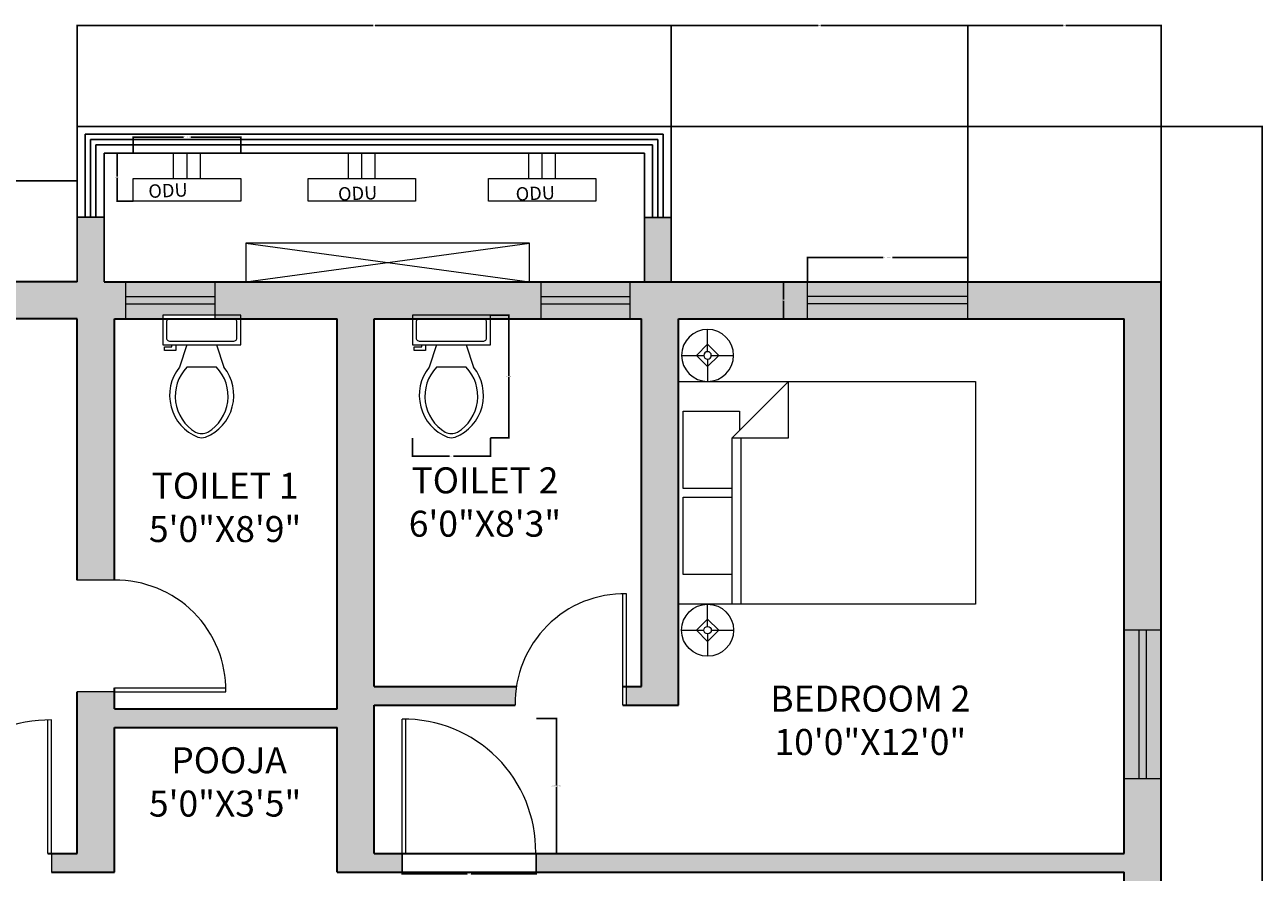
# Model space of a CAD drawing. Units: inches. Extents: x -382 to 250, y 518 to 1732.
# Tile 8 of 8: x -86 to 247, y 1504 to 1732. Entities that reach past the tile are written whole.
import ezdxf

# ---------------------------------------------------------------- set-up
doc = ezdxf.new("R2010")
doc.units = ezdxf.units.IN
doc.header["$MEASUREMENT"] = 0
for name, color, linetype, lineweight in [('A-ANNO-DIMS', 2, 'Continuous', 18), ('A-AREA-IDEN', 7, 'Continuous', 18), ('A-DOOR', 3, 'Continuous', 18), ('A-FLOR-EDGE', 7, 'Continuous', 25), ('A-FLOR-FIXT', 8, 'Continuous', 18), ('A-FLOR-SHFT', 8, 'Continuous', 18), ('A-FURN', 8, 'Continuous', 18), ('A-GLAZ', 4, 'Continuous', 18), ('A-WALL', 7, 'Continuous', 35), ('M-ANNO-TEXT', 7, 'Continuous', 13), ('M-HVAC-EQPM', 4, 'Continuous', 18)]:
    doc.layers.add(name, color=color, linetype=linetype, lineweight=lineweight)
doc.layers.add('A-GLAZ-PATT', color=143, linetype='Continuous', lineweight=13, true_color=0x7aafdf)
doc.layers.add('A-WALL-PATT', color=251, linetype='Continuous', lineweight=13, true_color=0x636466)
doc.styles.get("Standard").update_dxf_attribs({"font": 'arial.ttf'})
doc.dimstyles.get("Standard").update_dxf_attribs({"dimtxt": 0.18, "dimasz": 0.18, "dimexe": 0.18, "dimexo": 0.0625, "dimgap": 0.09, "dimtad": 0, "dimtih": 1, "dimtoh": 1, "dimdec": 4, "dimzin": 0, "dimdsep": 46, "dimtxsty": 'Standard', "dimcen": 0.09, "dimadec": 0, "dimazin": 0, "dimtfac": 1, "dimtdec": 4, "dimtofl": 0, "dimtmove": 0, "dimatfit": 3, "dimfxl": 1, "dimtolj": 1, "dimtzin": 0, "dimarcsym": 0})

# ---------------------------------------------------------------- blocks, each defined once
blk = doc.blocks.new('Bed - Queen')
for p, q in [((0, -80.00003), (0, 0)), ((0, 0), (59.99999, 0)), ((59.99999, 0), (59.99999, -80.00003)), ((7.99999, -1.2), (28.79998, -1.2)), ((7.99999, -14.4), (7.99999, -1.2)), ((28.79998, -1.2), (28.79998, -14.4)), ((31.19999, -1.2), (51.99999, -1.2)), ((31.19999, -14.4), (31.19999, -1.2)), ((51.99999, -1.2), (51.99999, -16.4)), ((0, -14.4), (44.8, -14.4)), ((59.99999, -29.6), (44.8, -14.4)), ((44.8, -14.4), (44.8, -29.6)), ((51.99999, -16.4), (46.79936, -16.4)), ((44.8, -16.8), (0, -16.8)), ((44.8, -29.6), (59.99999, -29.6)), ((59.99999, -80.00003), (0, -80.00003))]:
    blk.add_line(p, q)
blk = doc.blocks.new('Lamp - Table')
for p, q in [((0, 7), (0, 1)), ((-1, 0), (-7, 0)), ((0, 3), (-3, 0)), ((-3, 0), (0, -3)), ((3, 0), (0, 3)), ((0, -3), (3, 0)), ((1, 0), (7, 0)), ((0, -1), (0, -7))]:
    blk.add_line(p, q)
for radius in [7, 1]:
    blk.add_circle((0, 0), radius)
blk = doc.blocks.new('Toilet - top')
for p, q in [((9.5, -6), (9.5, -2)), ((-10, -8.5), (-8, -8.5)), ((-10, -9.5), (-10, -8.5)), ((-7, -9.5), (-10, -9.5)), ((-8, -8.5), (-8, -8)), ((-7, -8), (-7, -9.5)), ((-4, -8), (-6, -14)), ((4, -8), (6, -14)), ((4, -14), (-4, -14))]:
    blk.add_line(p, q)
blk.add_lwpolyline([(10.5, -8), (10.5, 0), (-10.5, 0), (-10.5, -8)], close=True)
for points in [[(-9.5, -2), (-9.5, -6)], [(8.5, -1), (-8.5, -1)], [(-8.5, -7), (8.5, -7)]]:
    blk.add_lwpolyline(points)
for centre, radius, start, end in [((-8.62, -1.88), 0.884, 81.8699, 188.1301), ((8.62, -1.88), 0.884, 351.8699, 98.1301), ((-8.62, -6.12), 0.884, 171.8699, 278.1301), ((8.62, -6.12), 0.884, 261.8699, 8.1301), ((3.52, -21.58), 12.17, 141.4691, 247.9714), ((4.2, -21.82), 11.33, 136.3677, 238.9468), ((-3.52, -21.58), 12.17, 292.0284, 38.5307), ((-4.2, -21.82), 11.33, 301.053, 43.6321), ((0, -27.88), 4, 245.7318, 294.2682), ((0, -29), 4, 254.8605, 285.1395)]:
    blk.add_arc(centre, radius, start, end)
blk = doc.blocks.new('WIN-43_2IN')
for p, q in [((0, 10), (0, 0)), ((43.2, 10), (43.2, 0)), ((0, 6), (43.2, 6)), ((0, 4), (43.2, 4))]:
    blk.add_line(p, q)
blk = doc.blocks.new('WIN-40IN')
for p, q in [((10, 40), (0, 40)), ((4, 40), (4, 0)), ((6, 40), (6, 0)), ((10, 0), (0, 0))]:
    blk.add_line(p, q)
blk = doc.blocks.new('WIN-24IN')
for p, q in [((0, 0), (0, 10)), ((24, 0), (24, 10)), ((0, 6), (24, 6)), ((0, 4), (24, 4))]:
    blk.add_line(p, q)
blk = doc.blocks.new('DOOR-SWING-36IN')
for p, q in [((-1, 0), (-1, 36)), ((0, 0), (0, 36))]:
    blk.add_line(p, q)
blk.add_arc((-0.5, 0.5), 35.5, 89.1931, 180.8069)
blk = doc.blocks.new('DOOR-SWING-30IN')
for p, q in [((0, 1), (30, 1)), ((0, 0), (30, 0))]:
    blk.add_line(p, q)
blk.add_arc((0.5, 0.5), 29.5, 359.029, 90.971)
blk = doc.blocks.new('ODU-LEDGE-MEDIUM')
for p, q in [((10.89, 6.17), (10.89, 12.93)), ((14.49, 6.17), (14.49, 12.93)), ((18.09, 6.17), (18.09, 12.93))]:
    blk.add_line(p, q)
blk.add_lwpolyline([(0, 6.17), (28.98, 6.17), (28.98, 0), (0, 0)], close=True)
blk = doc.blocks.new('DOOR-SWING-36IN-OFFSET')
for p, q in [((0, 0), (0, 36)), ((1, -0.22), (1, 36))]:
    blk.add_line(p, q)
blk.add_arc((0.5, 0.5), 35.5, 359.1931, 90.8069)
blk = doc.blocks.new('*D42')
at = {"layer": 'A-ANNO-DIMS', "color": 0, "lineweight": -2, "transparency": 16777216}
for p, q in [((39.13, 1654.07), (44.21, 1654.07)), ((44.03, 1653.89), (44.03, 1637.73)), ((44.03, 1621.2), (44.03, 1637.36)), ((39.13, 1621.02), (44.21, 1621.02))]:
    blk.add_line(p, q, dxfattribs=at)
at = {"layer": 'A-ANNO-DIMS', "color": 0, "transparency": 16777216}
for points in [[(44, 1653.89), (44.06, 1653.89), (44.03, 1654.07)], [(44, 1621.2), (44.06, 1621.2), (44.03, 1621.02)]]:
    blk.add_solid(points, dxfattribs=at)
at = {"layer": 'Defpoints', "color": 0, "transparency": 16777216}
for p in [(39.07, 1654.07), (44.03, 1654.07), (39.07, 1621.02)]:
    blk.add_point(p, dxfattribs=at)
at = {"layer": 'A-ANNO-DIMS', "color": 0, "transparency": 16777216, "insert": (44.03, 1637.55), "char_height": 0.18, "attachment_point": 5}
blk.add_mtext('\\A1;WC 33 TYP.', dxfattribs=at)
blk = doc.blocks.new('*D43')
at = {"layer": 'A-ANNO-DIMS', "color": 0, "lineweight": -2, "transparency": 16777216}
for p, q in [((18.07, 1620.96), (18.07, 1615.89)), ((39.07, 1620.96), (39.07, 1615.89)), ((18.25, 1616.07), (28.04, 1616.07)), ((38.89, 1616.07), (29.1, 1616.07))]:
    blk.add_line(p, q, dxfattribs=at)
at = {"layer": 'A-ANNO-DIMS', "color": 0, "transparency": 16777216}
for points in [[(18.25, 1616.1), (18.25, 1616.04), (18.07, 1616.07)], [(38.89, 1616.1), (38.89, 1616.04), (39.07, 1616.07)]]:
    blk.add_solid(points, dxfattribs=at)
at = {"layer": 'Defpoints', "color": 0, "transparency": 16777216}
for p in [(18.07, 1621.02), (39.07, 1621.02), (39.07, 1616.07)]:
    blk.add_point(p, dxfattribs=at)
at = {"layer": 'A-ANNO-DIMS', "color": 0, "transparency": 16777216, "insert": (28.57, 1616.07), "char_height": 0.18, "attachment_point": 5}
blk.add_mtext('\\A1;21 TYP.', dxfattribs=at)
blk = doc.blocks.new('*D52')
at = {"layer": 'A-ANNO-DIMS', "color": 0, "lineweight": -2, "transparency": 16777216}
for p, q in [((-57.14, 1697.73), (-57.14, 1702.19)), ((-56.96, 1702.01), (-43.64, 1702.01)), ((-28.34, 1702.01), (-41.66, 1702.01)), ((-28.16, 1697.73), (-28.16, 1702.19))]:
    blk.add_line(p, q, dxfattribs=at)
at = {"layer": 'A-ANNO-DIMS', "color": 0, "transparency": 16777216}
for points in [[(-56.96, 1702.04), (-56.96, 1701.98), (-57.14, 1702.01)], [(-28.34, 1702.04), (-28.34, 1701.98), (-28.16, 1702.01)]]:
    blk.add_solid(points, dxfattribs=at)
at = {"layer": 'Defpoints', "color": 0, "transparency": 16777216}
for p in [(-28.16, 1702.01), (-57.14, 1697.66), (-28.16, 1697.66)]:
    blk.add_point(p, dxfattribs=at)
at = {"layer": 'A-ANNO-DIMS', "color": 0, "transparency": 16777216, "insert": (-42.65, 1702.01), "char_height": 0.18, "attachment_point": 5}
blk.add_mtext('\\A1;ODU-M 29 TYP.', dxfattribs=at)
blk = doc.blocks.new('*D53')
at = {"layer": 'A-ANNO-DIMS', "color": 0, "lineweight": -2, "transparency": 16777216}
for p, q in [((-57.2, 1697.66), (-61.67, 1697.66)), ((-61.49, 1697.48), (-61.49, 1691.38)), ((-61.49, 1684.91), (-61.49, 1691.02)), ((-57.2, 1684.73), (-61.67, 1684.73))]:
    blk.add_line(p, q, dxfattribs=at)
at = {"layer": 'A-ANNO-DIMS', "color": 0, "transparency": 16777216}
for points in [[(-61.52, 1697.48), (-61.46, 1697.48), (-61.49, 1697.66)], [(-61.52, 1684.91), (-61.46, 1684.91), (-61.49, 1684.73)]]:
    blk.add_solid(points, dxfattribs=at)
at = {"layer": 'Defpoints', "color": 0, "transparency": 16777216}
for p in [(-61.49, 1697.66), (-57.14, 1697.66), (-57.14, 1684.73)]:
    blk.add_point(p, dxfattribs=at)
at = {"layer": 'A-ANNO-DIMS', "color": 0, "transparency": 16777216, "insert": (-61.49, 1691.2), "char_height": 0.18, "attachment_point": 5}
blk.add_mtext('\\A1;13 TYP.', dxfattribs=at)
blk = doc.blocks.new('*D62')
at = {"layer": 'A-ANNO-DIMS', "color": 0, "lineweight": -2, "transparency": 16777216}
for p, q in [((51.48, 1545.42), (57.05, 1545.42)), ((56.87, 1545.24), (56.87, 1527.43)), ((56.87, 1509.25), (56.87, 1527.06)), ((51.48, 1509.07), (57.05, 1509.07))]:
    blk.add_line(p, q, dxfattribs=at)
at = {"layer": 'A-ANNO-DIMS', "color": 0, "transparency": 16777216}
for points in [[(56.84, 1545.24), (56.9, 1545.24), (56.87, 1545.42)], [(56.84, 1509.25), (56.9, 1509.25), (56.87, 1509.07)]]:
    blk.add_solid(points, dxfattribs=at)
at = {"layer": 'Defpoints', "color": 0, "transparency": 16777216}
for p in [(51.42, 1545.42), (56.87, 1545.42), (51.42, 1509.07)]:
    blk.add_point(p, dxfattribs=at)
at = {"layer": 'A-ANNO-DIMS', "color": 0, "transparency": 16777216, "insert": (56.87, 1527.24), "char_height": 0.18, "attachment_point": 5}
blk.add_mtext('\\A1;OFFSET DOOR 36 TYP.', dxfattribs=at)
blk = doc.blocks.new('*D63')
at = {"layer": 'A-ANNO-DIMS', "color": 0, "lineweight": -2, "transparency": 16777216}
for p, q in [((15.29, 1509.01), (15.29, 1503.44)), ((51.42, 1509.01), (51.42, 1503.44)), ((15.47, 1503.62), (32.82, 1503.62)), ((51.24, 1503.62), (33.88, 1503.62))]:
    blk.add_line(p, q, dxfattribs=at)
at = {"layer": 'A-ANNO-DIMS', "color": 0, "transparency": 16777216}
for points in [[(15.47, 1503.65), (15.47, 1503.59), (15.29, 1503.62)], [(51.24, 1503.65), (51.24, 1503.59), (51.42, 1503.62)]]:
    blk.add_solid(points, dxfattribs=at)
at = {"layer": 'Defpoints', "color": 0, "transparency": 16777216}
for p in [(15.29, 1509.07), (51.42, 1509.07), (51.42, 1503.62)]:
    blk.add_point(p, dxfattribs=at)
at = {"layer": 'A-ANNO-DIMS', "color": 0, "transparency": 16777216, "insert": (33.35, 1503.62), "char_height": 0.18, "attachment_point": 5}
blk.add_mtext('\\A1;36 TYP.', dxfattribs=at)
blk = doc.blocks.new('*D68')
at = {"layer": 'A-ANNO-DIMS', "color": 0, "lineweight": -2, "transparency": 16777216}
for p, q in [((124.53, 1663.13), (124.53, 1669.73)), ((124.71, 1669.55), (144.89, 1669.55)), ((167.55, 1669.55), (147.37, 1669.55)), ((167.73, 1663.13), (167.73, 1669.73))]:
    blk.add_line(p, q, dxfattribs=at)
at = {"layer": 'A-ANNO-DIMS', "color": 0, "transparency": 16777216}
for points in [[(124.71, 1669.58), (124.71, 1669.52), (124.53, 1669.55)], [(167.55, 1669.58), (167.55, 1669.52), (167.73, 1669.55)]]:
    blk.add_solid(points, dxfattribs=at)
at = {"layer": 'Defpoints', "color": 0, "transparency": 16777216}
for p in [(124.53, 1669.55), (124.53, 1663.07), (167.73, 1663.07)]:
    blk.add_point(p, dxfattribs=at)
at = {"layer": 'A-ANNO-DIMS', "color": 0, "transparency": 16777216, "insert": (146.13, 1669.55), "char_height": 0.18, "attachment_point": 5}
blk.add_mtext('\\A1;WINDOW A 43 TYP.', dxfattribs=at)
blk = doc.blocks.new('*D69')
at = {"layer": 'A-ANNO-DIMS', "color": 0, "lineweight": -2, "transparency": 16777216}
for p, q in [((124.47, 1663.07), (117.87, 1663.07)), ((118.05, 1662.89), (118.05, 1658.25)), ((118.05, 1653.25), (118.05, 1657.89)), ((124.47, 1653.07), (117.87, 1653.07))]:
    blk.add_line(p, q, dxfattribs=at)
at = {"layer": 'A-ANNO-DIMS', "color": 0, "transparency": 16777216}
for points in [[(118.02, 1662.89), (118.08, 1662.89), (118.05, 1663.07)], [(118.02, 1653.25), (118.08, 1653.25), (118.05, 1653.07)]]:
    blk.add_solid(points, dxfattribs=at)
at = {"layer": 'Defpoints', "color": 0, "transparency": 16777216}
for p in [(124.53, 1663.07), (118.05, 1653.07), (124.53, 1653.07)]:
    blk.add_point(p, dxfattribs=at)
at = {"layer": 'A-ANNO-DIMS', "color": 0, "transparency": 16777216, "insert": (118.05, 1658.07), "char_height": 0.18, "attachment_point": 5}
blk.add_mtext('\\A1;10 TYP.', dxfattribs=at)
blk = doc.blocks.new('*D87')
at = {"layer": 'A-ANNO-DIMS', "color": 0, "lineweight": -2, "transparency": 16777216}
for p, q in [((87.85, 1704.87), (247.16, 1704.87)), ((246.98, 1704.69), (246.98, 1437.22)), ((246.98, 1169.38), (246.98, 1436.85)), ((82.25, 1169.2), (247.16, 1169.2))]:
    blk.add_line(p, q, dxfattribs=at)
at = {"layer": 'A-ANNO-DIMS', "color": 0, "transparency": 16777216}
for points in [[(246.95, 1704.69), (247.01, 1704.69), (246.98, 1704.87)], [(246.95, 1169.38), (247.01, 1169.38), (246.98, 1169.2)]]:
    blk.add_solid(points, dxfattribs=at)
at = {"layer": 'Defpoints', "color": 0, "transparency": 16777216}
for p in [(87.78, 1704.87), (246.98, 1704.87), (82.19, 1169.2)]:
    blk.add_point(p, dxfattribs=at)
at = {"layer": 'A-ANNO-DIMS', "color": 0, "transparency": 16777216, "insert": (246.98, 1437.03), "char_height": 0.18, "attachment_point": 5}
blk.add_mtext('\\A1;535.7', dxfattribs=at)
blk = doc.blocks.new('*D88')
at = {"layer": 'A-ANNO-DIMS', "color": 0, "lineweight": -2, "transparency": 16777216}
for p, q in [((-202.22, 1663.13), (-202.22, 1690.45)), ((-202.04, 1690.27), (-137.5, 1690.27)), ((-72.4, 1690.27), (-136.93, 1690.27)), ((-72.22, 1663.13), (-72.22, 1690.45))]:
    blk.add_line(p, q, dxfattribs=at)
at = {"layer": 'A-ANNO-DIMS', "color": 0, "transparency": 16777216}
for points in [[(-202.04, 1690.3), (-202.04, 1690.24), (-202.22, 1690.27)], [(-72.4, 1690.3), (-72.4, 1690.24), (-72.22, 1690.27)]]:
    blk.add_solid(points, dxfattribs=at)
at = {"layer": 'Defpoints', "color": 0, "transparency": 16777216}
for p in [(-72.22, 1690.27), (-202.22, 1663.07), (-72.22, 1663.07)]:
    blk.add_point(p, dxfattribs=at)
at = {"layer": 'A-ANNO-DIMS', "color": 0, "transparency": 16777216, "insert": (-137.22, 1690.27), "char_height": 0.18, "attachment_point": 5}
blk.add_mtext('\\A1;130', dxfattribs=at)
blk = doc.blocks.new('*D89')
at = {"layer": 'A-ANNO-DIMS', "color": 0, "lineweight": -2, "transparency": 16777216}
for p, q in [((-72.22, 1704.93), (-72.22, 1732.25)), ((-72.04, 1732.07), (7.5, 1732.07)), ((87.6, 1732.07), (8.07, 1732.07)), ((87.78, 1704.93), (87.78, 1732.25))]:
    blk.add_line(p, q, dxfattribs=at)
at = {"layer": 'A-ANNO-DIMS', "color": 0, "transparency": 16777216}
for points in [[(-72.04, 1732.1), (-72.04, 1732.04), (-72.22, 1732.07)], [(87.6, 1732.1), (87.6, 1732.04), (87.78, 1732.07)]]:
    blk.add_solid(points, dxfattribs=at)
at = {"layer": 'Defpoints', "color": 0, "transparency": 16777216}
for p in [(87.78, 1732.07), (-72.22, 1704.87), (87.78, 1704.87)]:
    blk.add_point(p, dxfattribs=at)
at = {"layer": 'A-ANNO-DIMS', "color": 0, "transparency": 16777216, "insert": (7.78, 1732.07), "char_height": 0.18, "attachment_point": 5}
blk.add_mtext('\\A1;160', dxfattribs=at)
blk = doc.blocks.new('*D90')
at = {"layer": 'A-ANNO-DIMS', "color": 0, "lineweight": -2, "transparency": 16777216}
for p, q in [((87.78, 1704.93), (87.78, 1732.25)), ((87.96, 1732.07), (127.36, 1732.07)), ((167.55, 1732.07), (128.15, 1732.07)), ((167.73, 1663.13), (167.73, 1732.25))]:
    blk.add_line(p, q, dxfattribs=at)
at = {"layer": 'A-ANNO-DIMS', "color": 0, "transparency": 16777216}
for points in [[(87.96, 1732.1), (87.96, 1732.04), (87.78, 1732.07)], [(167.55, 1732.1), (167.55, 1732.04), (167.73, 1732.07)]]:
    blk.add_solid(points, dxfattribs=at)
at = {"layer": 'Defpoints', "color": 0, "transparency": 16777216}
for p in [(167.73, 1732.07), (87.78, 1704.87), (167.73, 1663.07)]:
    blk.add_point(p, dxfattribs=at)
at = {"layer": 'A-ANNO-DIMS', "color": 0, "transparency": 16777216, "insert": (127.76, 1732.07), "char_height": 0.18, "attachment_point": 5}
blk.add_mtext('\\A1;79.95', dxfattribs=at)
blk = doc.blocks.new('*D96')
at = {"layer": 'A-ANNO-DIMS', "color": 0, "lineweight": -2, "transparency": 16777216}
for p, q in [((167.73, 1663.13), (167.73, 1732.25)), ((167.91, 1732.07), (193.36, 1732.07)), ((219.6, 1732.07), (194.15, 1732.07)), ((219.78, 1663.13), (219.78, 1732.25))]:
    blk.add_line(p, q, dxfattribs=at)
at = {"layer": 'A-ANNO-DIMS', "color": 0, "transparency": 16777216}
for points in [[(167.91, 1732.1), (167.91, 1732.04), (167.73, 1732.07)], [(219.6, 1732.1), (219.6, 1732.04), (219.78, 1732.07)]]:
    blk.add_solid(points, dxfattribs=at)
at = {"layer": 'Defpoints', "color": 0, "transparency": 16777216}
for p in [(219.78, 1732.07), (167.73, 1663.07), (219.78, 1663.07)]:
    blk.add_point(p, dxfattribs=at)
at = {"layer": 'A-ANNO-DIMS', "color": 0, "transparency": 16777216, "insert": (193.76, 1732.07), "char_height": 0.18, "attachment_point": 5}
blk.add_mtext('\\A1;52.05', dxfattribs=at)

msp = doc.modelspace()

# ---------------------------------------------------------------- hatches: boundary and pattern name
at = {"layer": 'A-GLAZ-PATT'}
h = msp.add_hatch(color=256, dxfattribs=at)
h.dxf.hatch_style = 1
h.paths.add_polyline_path([(-35.1064, 1663.0687), (-59.1064, 1663.0687), (-59.1064, 1659.0687), (-35.1064, 1659.0687)])
h = msp.add_hatch(color=256, dxfattribs=at)
h.dxf.hatch_style = 1
h.paths.add_polyline_path([(76.7201, 1663.0687), (52.7201, 1663.0687), (52.7201, 1659.0687), (76.7201, 1659.0687)])
h = msp.add_hatch(color=256, dxfattribs=at)
h.dxf.hatch_style = 1
h.paths.add_polyline_path([(167.7319, 1663.0687), (149.785, 1663.0687), (124.5319, 1663.0687), (124.5319, 1659.0687), (167.7319, 1659.0687)])
h = msp.add_hatch(color=256, dxfattribs=at)
h.dxf.hatch_style = 1
h.paths.add_polyline_path([(-35.1064, 1659.0687), (-59.1064, 1659.0687), (-59.1064, 1657.0687), (-35.1064, 1657.0687)])
h = msp.add_hatch(color=256, dxfattribs=at)
h.dxf.hatch_style = 1
h.paths.add_polyline_path([(76.7201, 1659.0687), (52.7201, 1659.0687), (52.7201, 1657.0687), (76.7201, 1657.0687)])
h = msp.add_hatch(color=256, dxfattribs=at)
h.dxf.hatch_style = 1
h.paths.add_polyline_path([(167.7319, 1659.0687), (124.5319, 1659.0687), (124.5319, 1657.0687), (167.7319, 1657.0687)])
h = msp.add_hatch(color=256, dxfattribs=at)
h.dxf.hatch_style = 1
h.paths.add_polyline_path([(-35.1064, 1657.0687), (-59.1064, 1657.0687), (-59.1064, 1653.0687), (-49.1947, 1653.0687), (-49.1947, 1654.0687), (-35.1064, 1654.0687)])
h = msp.add_hatch(color=256, dxfattribs=at)
h.dxf.hatch_style = 1
h.paths.add_polyline_path([(76.7201, 1657.0687), (52.7201, 1657.0687), (52.7201, 1653.0687), (76.7201, 1653.0687)])
h = msp.add_hatch(color=256, dxfattribs=at)
h.dxf.hatch_style = 1
h.paths.add_polyline_path([(167.7319, 1657.0687), (124.5319, 1657.0687), (124.5319, 1653.0687), (167.7319, 1653.0687)])
h = msp.add_hatch(color=256, dxfattribs=at)
h.dxf.hatch_style = 1
h.paths.add_polyline_path([(213.785, 1569.2079), (209.785, 1569.2079), (209.785, 1529.2079), (213.785, 1529.2079)])
h = msp.add_hatch(color=256, dxfattribs=at)
h.dxf.hatch_style = 1
h.paths.add_polyline_path([(215.785, 1569.2079), (213.785, 1569.2079), (213.785, 1529.2079), (215.785, 1529.2079)])
h = msp.add_hatch(color=256, dxfattribs=at)
h.dxf.hatch_style = 1
h.paths.add_polyline_path([(219.785, 1569.2079), (215.785, 1569.2079), (215.785, 1529.2079), (219.785, 1529.2079)])
at = {"layer": 'A-WALL-PATT'}
h = msp.add_hatch(color=256, dxfattribs=at)
h.dxf.hatch_style = 1
h.paths.add_polyline_path([(-62.215, 1653.0687), (-59.1064, 1653.0687), (-59.1064, 1663.0687), (-65.0078, 1663.0687), (-65.0078, 1680.4388), (-72.215, 1680.4388), (-72.215, 1663.0687), (-113.7732, 1663.0687), (-113.7732, 1653.0687), (-72.215, 1653.0687), (-72.215, 1582.6793), (-62.215, 1582.6793)])
h = msp.add_hatch(color=256, dxfattribs=at)
h.dxf.hatch_style = 1
h.paths.add_polyline_path([(87.785, 1680.366), (80.5778, 1680.366), (80.5778, 1663.0687), (87.785, 1663.0687)])
h = msp.add_hatch(color=256, dxfattribs=at)
h.dxf.hatch_style = 1
h.paths.add_polyline_path([(-62.215, 1543.0687), (-2.215, 1543.0687), (-2.215, 1504.0687), (15.2853, 1504.0687), (15.2853, 1509.0687), (7.785, 1509.0687), (7.785, 1549.0687), (45.742, 1549.0687, -0.04254204), (46.083, 1554.0687), (7.785, 1554.0687), (7.785, 1653.0687), (52.7201, 1653.0687), (52.7201, 1663.0687), (7.785, 1663.0687), (-26.8096, 1663.0687), (-35.1064, 1663.0687), (-35.1064, 1653.0687), (-2.215, 1653.0687), (-2.215, 1548.0687), (-62.215, 1548.0687), (-62.215, 1552.6793), (-72.215, 1552.6793), (-72.215, 1509.0687), (-79.1204, 1509.0687), (-79.1204, 1504.0687), (-62.215, 1504.0687)])
h = msp.add_hatch(color=256, dxfattribs=at)
h.dxf.hatch_style = 1
h.paths.add_polyline_path([(89.785, 1653.0687), (124.5319, 1653.0687), (124.5319, 1663.0687), (89.785, 1663.0687), (76.7201, 1663.0687), (76.7201, 1653.0687), (79.785, 1653.0687), (79.785, 1554.0687), (75.742, 1554.0687), (75.742, 1549.0687), (89.785, 1549.0687)])
h = msp.add_hatch(color=256, dxfattribs=at)
h.dxf.hatch_style = 1
h.paths.add_polyline_path([(219.785, 1663.0687), (167.7319, 1663.0687), (167.7319, 1653.0687), (209.785, 1653.0687), (209.785, 1569.2079), (219.785, 1569.2079)])
h = msp.add_hatch(color=256, dxfattribs=at)
h.dxf.hatch_style = 1
h.paths.add_polyline_path([(219.785, 1529.2079), (209.785, 1529.2079), (209.785, 1509.0687), (51.2853, 1509.0687), (51.2853, 1504.0687), (209.785, 1504.0687), (209.785, 1489.835), (219.785, 1489.835)])

# ---------------------------------------------------------------- linework, layer by layer
at = {"layer": 'A-DOOR'}
for p, q in [((-62.215, 1582.6793), (-72.215, 1582.6793)), ((-62.215, 1552.6793), (-72.215, 1552.6793)), ((-79.1204, 1509.0687), (-79.1204, 1504.0687)), ((15.2853, 1509.2855), (15.2853, 1504.0687)), ((51.2853, 1509.2855), (51.2853, 1504.0687))]:
    msp.add_line(p, q, dxfattribs=at)
at = {"layer": 'A-FLOR-EDGE'}
for p, q in [((-72.215, 1663.0687), (-72.215, 1704.8705)), ((-72.215, 1704.8705), (87.785, 1704.8705)), ((-70.0529, 1680.366), (-70.0529, 1702.7914)), ((85.6228, 1702.7914), (-70.0529, 1702.7914)), ((85.6228, 1680.366), (85.6228, 1702.7914)), ((87.785, 1663.0687), (87.785, 1704.8705)), ((-68.6114, 1680.366), (-68.6114, 1701.35)), ((84.1814, 1701.35), (-68.6114, 1701.35)), ((-67.17, 1680.366), (-67.17, 1699.9085)), ((82.7399, 1699.9085), (-67.17, 1699.9085)), ((82.7399, 1680.366), (82.7399, 1699.9085)), ((84.1814, 1680.366), (84.1814, 1701.35)), ((-65.0078, 1663.0687), (-65.0078, 1697.6633)), ((-65.0078, 1697.6633), (80.5778, 1697.6633)), ((80.5778, 1663.0687), (80.5778, 1697.6633)), ((-72.215, 1680.4388), (-65.0078, 1680.4388)), ((80.5778, 1680.366), (87.785, 1680.366))]:
    msp.add_line(p, q, dxfattribs=at)
at = {"layer": 'A-FLOR-SHFT'}
for p, q in [((-26.8096, 1663.0687), (49.5868, 1673.4832)), ((-26.8096, 1673.4832), (49.5868, 1663.0687))]:
    msp.add_line(p, q, dxfattribs=at)
msp.add_lwpolyline([(-26.8096, 1663.0687), (49.5868, 1663.0687), (49.5868, 1673.4832), (-26.8096, 1673.4832)], close=True, dxfattribs=at)
at = {"layer": 'A-WALL'}
for p, q in [((-72.215, 1663.0687), (-202.215, 1663.0687)), ((-65.0078, 1663.0687), (7.785, 1663.0687)), ((7.785, 1663.0687), (89.785, 1663.0687)), ((89.785, 1663.0687), (150.3243, 1663.0687)), ((149.785, 1663.0687), (219.785, 1663.0687)), ((219.785, 1489.835), (219.785, 1663.0687)), ((-72.215, 1653.0687), (-192.215, 1653.0687)), ((-72.215, 1582.6793), (-72.215, 1653.0687)), ((-62.215, 1653.0687), (-2.215, 1653.0687)), ((-62.215, 1582.6793), (-62.215, 1653.0687)), ((-2.215, 1548.0687), (-2.215, 1653.0687)), ((7.785, 1653.0687), (79.785, 1653.0687)), ((7.785, 1554.0687), (7.785, 1653.0687)), ((79.785, 1554.0687), (79.785, 1653.0687)), ((89.785, 1549.0687), (89.785, 1653.0687)), ((89.785, 1653.0687), (209.785, 1653.0687)), ((209.785, 1509.0687), (209.785, 1653.0687)), ((-72.215, 1509.0687), (-72.215, 1552.6793)), ((-62.215, 1548.0687), (-62.215, 1553.6793)), ((7.785, 1554.0687), (46.083, 1554.0687)), ((74.742, 1554.0687), (79.785, 1554.0687)), ((7.785, 1509.0687), (7.785, 1549.0687)), ((7.785, 1549.0687), (45.742, 1549.0687)), ((74.742, 1549.0687), (89.785, 1549.0687)), ((-62.215, 1548.0687), (-2.215, 1548.0687)), ((-62.215, 1504.0687), (-62.215, 1543.0687)), ((-62.215, 1543.0687), (-2.215, 1543.0687)), ((-2.215, 1504.0687), (-2.215, 1543.0687)), ((-80.1204, 1509.0687), (-72.215, 1509.0687)), ((7.785, 1509.0687), (209.785, 1509.0687)), ((-79.1204, 1504.0687), (-62.215, 1504.0687)), ((-2.215, 1504.0687), (209.785, 1504.0687)), ((209.785, 1488.835), (209.785, 1504.0687))]:
    msp.add_line(p, q, dxfattribs=at)
at = {"layer": 'M-HVAC-EQPM'}
msp.add_lwpolyline([(-10.0519, 1690.9042), (18.9263, 1690.9042), (18.9263, 1684.7324), (-10.0519, 1684.7324)], close=True, dxfattribs=at)

# ---------------------------------------------------------------- block references
at = {"layer": 'A-DOOR'}
for name, p in [('DOOR-SWING-30IN', (-62.215, 1552.6793)), ('DOOR-SWING-36IN', (-79.1204, 1509.0687)), ('DOOR-SWING-36IN-OFFSET', (15.2853, 1509.2855))]:
    msp.add_blockref(name, p, dxfattribs=at)
at = {"layer": 'A-DOOR', "rotation": 89.99999999999991}
msp.add_blockref('DOOR-SWING-30IN', (75.742, 1549.0687), dxfattribs=at)
at = {"layer": 'A-FLOR-FIXT'}
for p in [(-38.6947, 1654.0687), (28.572, 1654.0687)]:
    msp.add_blockref('Toilet - top', p, dxfattribs=at)
at = {"layer": 'A-FURN', "xscale": -1, "rotation": 90}
msp.add_blockref('Lamp - Table', (97.5964, 1643.2304), dxfattribs=at)
at = {"layer": 'A-FURN', "rotation": 90}
for name, p in [('Bed - Queen', (89.785, 1576.2304)), ('Lamp - Table', (97.5964, 1569.2304))]:
    msp.add_blockref(name, p, dxfattribs=at)
at = {"layer": 'A-GLAZ'}
for name, p in [('WIN-24IN', (-59.106, 1653.069)), ('WIN-24IN', (52.7205, 1653.069)), ('WIN-40IN', (209.785, 1529.2076))]:
    msp.add_blockref(name, p, dxfattribs=at)
at = {"layer": 'A-GLAZ', "rotation": 180}
msp.add_blockref('WIN-43_2IN', (167.7319, 1663.0684), dxfattribs=at)
at = {"layer": 'M-HVAC-EQPM'}
for p in [(-57.142, 1684.732), (-10.0524, 1684.732), (38.5288, 1684.732)]:
    msp.add_blockref('ODU-LEDGE-MEDIUM', p, dxfattribs=at)

# ---------------------------------------------------------------- texts
at = {"layer": 'A-AREA-IDEN', "char_height": 7, "attachment_point": 1}
for s, insert in [('\\pxqc;TOILET 1\\P5\'0"X8\'9"', (-72.215, 1611.639)), ('\\pxqc;TOILET 2\\P6\'0"X8\'3"', (-2.215, 1613.0787)), ('\\pxqc;BEDROOM 2\\P10\'0"X12\'0"', (101.6167, 1554.3105)), ('\\pxqc; POOJA\\P5\'0"X3\'5"', (-72.215, 1537.7147))]:
    msp.add_mtext_dynamic_manual_height_columns(s, width=79.656175, gutter_width=1, heights=[0], dxfattribs=dict(at, insert=insert))
at = {"layer": 'M-ANNO-TEXT', "char_height": 3.6036, "attachment_point": 1, "rotation": 2.33497}
for insert in [(-53.134, 1689.214), (-2.0402, 1688.4582), (45.8236, 1688.4582)]:
    msp.add_mtext_dynamic_manual_height_columns('ODU', width=9.836639, gutter_width=0.7207, heights=[0], dxfattribs=dict(at, insert=insert))

# ---------------------------------------------------------------- dimensions: what is measured, and where the dimension line sits
at = {"layer": 'A-ANNO-DIMS'}
for base, p1, p2, override, picture, middle in [((87.785, 1732.0705), (-72.215, 1704.8705), (87.785, 1704.8705), {"dimdec": 0, "dimlfac": 1, "dimrnd": 0, "dimzin": 0, "dimdsep": 46, "dimlunit": 2}, '*D89', (7.785, 1732.0705)), ((167.7319, 1732.0705), (87.785, 1704.8705), (167.7319, 1663.0687), {"dimdec": 2, "dimlfac": 1, "dimrnd": 0, "dimzin": 0, "dimdsep": 46, "dimlunit": 2}, '*D90', (127.7584, 1732.0705)), ((219.785, 1732.0705), (167.7319, 1663.0687), (219.785, 1663.0687), {"dimdec": 2, "dimlfac": 1, "dimrnd": 0, "dimzin": 0, "dimdsep": 46, "dimlunit": 2}, '*D96', (193.7584, 1732.0705)), ((-72.215, 1690.2687), (-202.215, 1663.0687), (-72.215, 1663.0687), {"dimdec": 0, "dimlfac": 1, "dimrnd": 0, "dimzin": 0, "dimdsep": 46, "dimlunit": 2}, '*D88', (-137.215, 1690.2687))]:
    dim = msp.add_linear_dim(base=base, p1=p1, p2=p2, dimstyle='Standard', override=override, dxfattribs=at)
    dim.commit()
    dim.dimension.update_dxf_attribs({"geometry": picture, "text_midpoint": middle})
for base, p1, p2, text, picture, middle in [((-28.1633, 1702.01), (-57.1416, 1697.6633), (-28.1633, 1697.6633), 'ODU-M <> TYP.', '*D52', (-42.6525, 1702.01)), ((39.072, 1616.0655), (18.072, 1621.0225), (39.072, 1621.0225), '<> TYP.', '*D43', (28.572, 1616.0655)), ((51.4204, 1503.6159), (15.2853, 1509.0687), (51.4204, 1509.0687), '<> TYP.', '*D63', (33.3528, 1503.6159))]:
    dim = msp.add_linear_dim(base=base, p1=p1, p2=p2, text=text, dimstyle='Standard', override={"dimdec": 0, "dimlfac": 1, "dimrnd": 0, "dimzin": 0, "dimdsep": 46, "dimlunit": 2}, dxfattribs=at)
    dim.commit()
    dim.dimension.update_dxf_attribs({"geometry": picture, "text_midpoint": middle})
dim = msp.add_linear_dim(base=(246.985, 1704.8705), p1=(82.1869, 1169.1977), p2=(87.785, 1704.8705), angle=90, dimstyle='Standard', override={"dimdec": 1, "dimlfac": 1, "dimrnd": 0, "dimzin": 0, "dimdsep": 46, "dimlunit": 2}, dxfattribs=at)
dim.commit()
dim.dimension.update_dxf_attribs({"geometry": '*D87', "text_midpoint": (246.985, 1437.0341)})
for base, p1, p2, angle, text, picture, middle in [((-61.4883, 1697.6633), (-57.1416, 1684.7324), (-57.1416, 1697.6633), 90, '<> TYP.', '*D53', (-61.4883, 1691.1978)), ((124.5319, 1669.5487), (167.7319, 1663.0687), (124.5319, 1663.0687), 180, 'WINDOW A <> TYP.', '*D68', (146.1319, 1669.5487)), ((118.0519, 1653.0687), (124.5319, 1663.0687), (124.5319, 1653.0687), 270, '<> TYP.', '*D69', (118.0519, 1658.0687)), ((44.0289, 1654.0687), (39.072, 1621.0225), (39.072, 1654.0687), 90, 'WC <> TYP.', '*D42', (44.0289, 1637.5456)), ((56.8732, 1545.4206), (51.4204, 1509.0687), (51.4204, 1545.4206), 90, 'OFFSET DOOR <> TYP.', '*D62', (56.8732, 1527.2446))]:
    dim = msp.add_linear_dim(base=base, p1=p1, p2=p2, angle=angle, text=text, dimstyle='Standard', override={"dimdec": 0, "dimlfac": 1, "dimrnd": 0, "dimzin": 0, "dimdsep": 46, "dimlunit": 2}, dxfattribs=at)
    dim.commit()
    dim.dimension.update_dxf_attribs({"geometry": picture, "text_midpoint": middle})

doc.saveas('drawing.dxf')
